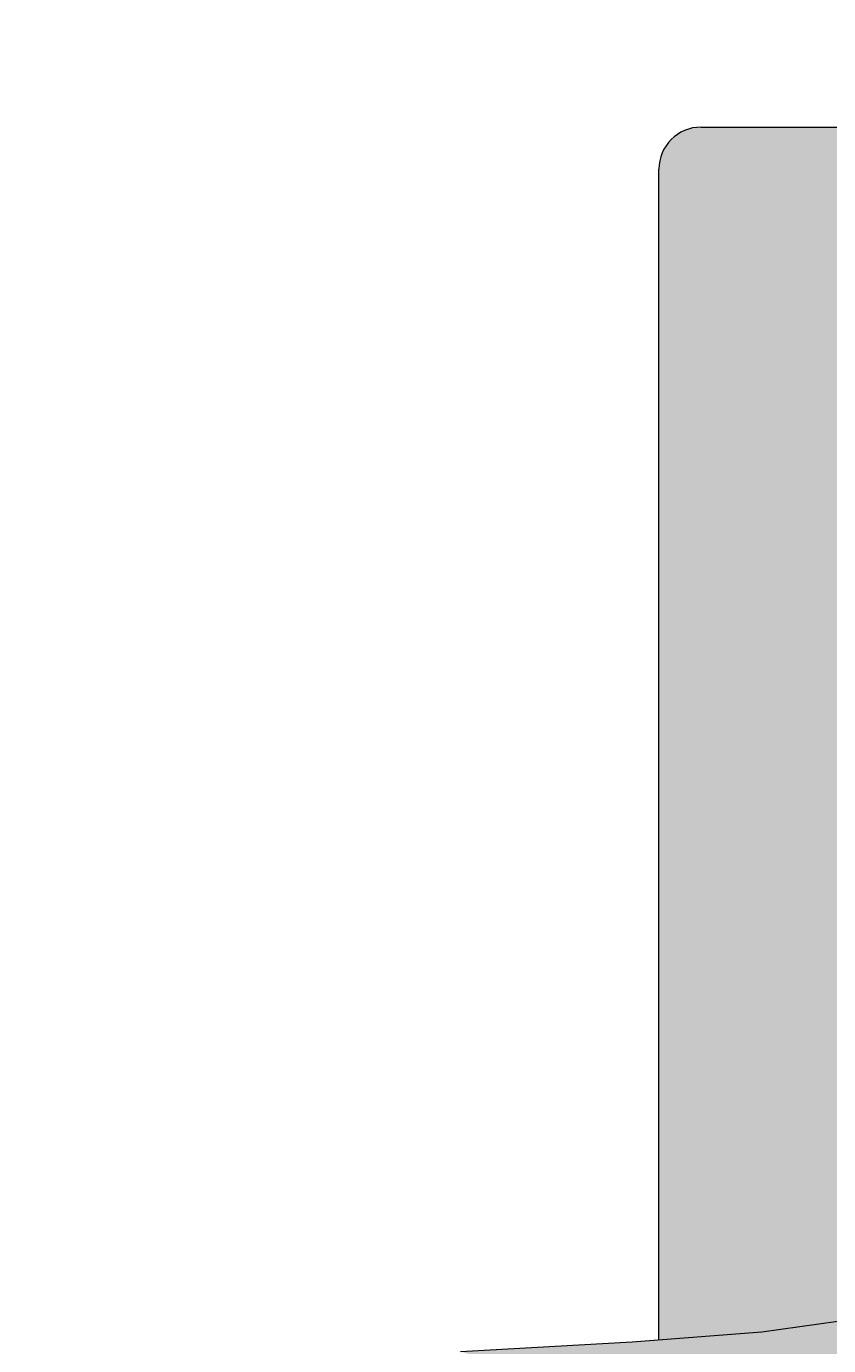
# Model space of a CAD drawing. Units: millimetres. Extents: x 27017497 to 27018854, y 7058029 to 7059154.
# Tile 73 of 91: x 27018360 to 27018390, y 7058174 to 7058224. Entities that reach past the tile are written whole.
import ezdxf

# ---------------------------------------------------------------- set-up
doc = ezdxf.new("R2010")
doc.units = ezdxf.units.MM
doc.layers.add('A-ANNO-DIMS', color=2, linetype='Continuous', lineweight=18)
doc.layers.add('A-FURN', color=8, linetype='Continuous', lineweight=18)
doc.layers.add('A-FURN-PATT', color=177, linetype='Continuous', lineweight=13, true_color=0x293189)
doc.styles.get("Standard").update_dxf_attribs({"font": 'arial.ttf'})
doc.dimstyles.get("Standard").update_dxf_attribs({"dimtxt": 0.18, "dimasz": 0.18, "dimexe": 0.18, "dimexo": 0.0625, "dimgap": 0.09, "dimtad": 0, "dimtih": 1, "dimtoh": 1, "dimdec": 4, "dimzin": 0, "dimdsep": 46, "dimtxsty": 'Standard', "dimcen": 0.09, "dimadec": 0, "dimazin": 0, "dimtfac": 1, "dimtdec": 4, "dimtofl": 0, "dimtmove": 0, "dimatfit": 3, "dimfxl": 1, "dimtolj": 1, "dimtzin": 0, "dimarcsym": 0})

# ---------------------------------------------------------------- blocks, each defined once
blk = doc.blocks.new('CAMMAT')
for p, q in [((0.65, -0.8204), (0.65, -1.93)), ((0.61, -1.97), (-0.61, -1.97))]:
    blk.add_line(p, q)
blk.add_lwpolyline([(0.8382, -0.8093), (0.6753, -0.8185), (0.5522, -0.828), (0.4622, -0.8406), (0.399, -0.8591), (0.356, -0.8862), (0.3267, -0.9248), (0.3046, -0.9777), (0.2832, -1.0476)])
blk.add_arc((0.61, -1.93), 0.04, 270, 360)
blk = doc.blocks.new('*D47')
at = {"layer": 'A-ANNO-DIMS', "color": 0, "lineweight": -2, "transparency": 16777216}
for p, q in [((27017561.166, 7058294.35), (27017561.166, 7058028.6)), ((27018790.606, 7058294.35), (27018790.606, 7058028.6)), ((27017561.346, 7058028.78), (27018175.431, 7058028.78)), ((27018790.426, 7058028.78), (27018176.341, 7058028.78))]:
    blk.add_line(p, q, dxfattribs=at)
at = {"layer": 'A-ANNO-DIMS', "color": 0, "transparency": 16777216}
for points in [[(27017561.346, 7058028.81), (27017561.346, 7058028.75), (27017561.166, 7058028.78)], [(27018790.426, 7058028.81), (27018790.426, 7058028.75), (27018790.606, 7058028.78)]]:
    blk.add_solid(points, dxfattribs=at)
at = {"layer": 'Defpoints', "color": 0, "transparency": 16777216}
for p in [(27017561.166, 7058294.412), (27018790.606, 7058294.412), (27018790.606, 7058028.78)]:
    blk.add_point(p, dxfattribs=at)
at = {"layer": 'A-ANNO-DIMS', "color": 0, "transparency": 16777216, "insert": (27018175.886, 7058028.78), "char_height": 0.18, "attachment_point": 5}
blk.add_mtext('\\A1;1229.4', dxfattribs=at)
blk = doc.blocks.new('*D48')
at = {"layer": 'A-ANNO-DIMS', "color": 0, "lineweight": -2, "transparency": 16777216}
for p, q in [((27018463.498, 7058622.912), (27017497.536, 7058622.912)), ((27017497.716, 7058622.732), (27017497.716, 7058357.753)), ((27017497.716, 7058092.41), (27017497.716, 7058357.389)), ((27018555.129, 7058092.23), (27017497.536, 7058092.23))]:
    blk.add_line(p, q, dxfattribs=at)
at = {"layer": 'A-ANNO-DIMS', "color": 0, "transparency": 16777216}
for points in [[(27017497.686, 7058622.732), (27017497.746, 7058622.732), (27017497.716, 7058622.912)], [(27017497.686, 7058092.41), (27017497.746, 7058092.41), (27017497.716, 7058092.23)]]:
    blk.add_solid(points, dxfattribs=at)
at = {"layer": 'Defpoints', "color": 0, "transparency": 16777216}
for p in [(27018463.561, 7058622.912), (27017497.716, 7058092.23), (27018555.192, 7058092.23)]:
    blk.add_point(p, dxfattribs=at)
at = {"layer": 'A-ANNO-DIMS', "color": 0, "transparency": 16777216, "insert": (27017497.716, 7058357.571), "char_height": 0.18, "attachment_point": 5}
blk.add_mtext('\\A1;530.7', dxfattribs=at)

msp = doc.modelspace()

# ---------------------------------------------------------------- hatches: boundary and pattern name
at = {"layer": 'A-FURN-PATT'}
h = msp.add_hatch(color=256, dxfattribs=at)
h.dxf.hatch_style = 1
h.paths.add_polyline_path([(27018435.86, 7058218.784, 0.414214), (27018434.267, 7058220.377), (27018385.674, 7058220.377, 0.414214), (27018384.081, 7058218.784), (27018384.081, 7058174.59), (27018387.977, 7058174.891), (27018391.56, 7058175.393), (27018394.078, 7058176.128), (27018395.791, 7058177.21), (27018396.958, 7058178.748), (27018397.838, 7058180.854), (27018398.69, 7058183.639), (27018399.293, 7058180.835), (27018399.836, 7058178.594), (27018400.426, 7058176.691), (27018401.17, 7058174.899), (27018402.177, 7058172.991), (27018403.552, 7058170.741), (27018405.403, 7058167.922), (27018407.838, 7058164.308), (27018410.273, 7058167.922), (27018412.124, 7058170.741), (27018413.499, 7058172.991), (27018414.506, 7058174.899), (27018415.25, 7058176.691), (27018415.84, 7058178.594), (27018416.383, 7058180.835), (27018416.986, 7058183.639), (27018417.838, 7058180.854), (27018418.718, 7058178.748), (27018419.885, 7058177.21), (27018421.598, 7058176.128), (27018424.116, 7058175.393), (27018427.699, 7058174.891), (27018432.604, 7058174.513), (27018435.86, 7058174.329)])
h.paths.add_polyline_path([(27018439.093, 7058174.146), (27018432.604, 7058174.513), (27018427.699, 7058174.891), (27018424.116, 7058175.393), (27018421.598, 7058176.128), (27018419.885, 7058177.21), (27018418.718, 7058178.748), (27018417.838, 7058180.854), (27018416.986, 7058183.639), (27018416.383, 7058180.835), (27018415.84, 7058178.594), (27018415.25, 7058176.691), (27018414.506, 7058174.899), (27018413.499, 7058172.991), (27018412.124, 7058170.741), (27018410.273, 7058167.922), (27018407.838, 7058164.308)])
h.paths.add_polyline_path([(27018403.552, 7058170.741), (27018402.177, 7058172.991), (27018401.17, 7058174.899), (27018400.426, 7058176.691), (27018399.836, 7058178.594), (27018399.293, 7058180.835), (27018398.69, 7058183.639), (27018397.838, 7058180.854), (27018396.958, 7058178.748), (27018395.791, 7058177.21), (27018394.078, 7058176.128), (27018391.56, 7058175.393), (27018387.977, 7058174.891), (27018383.071, 7058174.513), (27018376.583, 7058174.146), (27018407.838, 7058164.308), (27018405.403, 7058167.922)])
h.paths.add_polyline_path([(27018437.469, 7058173.635), (27018407.838, 7058164.308), (27018382.784, 7058172.194), (27018382.784, 7058162.502), (27018437.469, 7058162.502)])
h.paths.add_polyline_path([(27018435.86, 7058162.502), (27018384.081, 7058162.502), (27018384.081, 7058146.294, 0.414214), (27018385.674, 7058144.7), (27018434.267, 7058144.7, 0.414214), (27018435.86, 7058146.294)])
h.paths.add_polyline_path([(27018407.684, 7058159.418, -0.41419), (27018408.879, 7058158.223), (27018408.879, 7058148.664, -0.414237), (27018407.684, 7058147.469), (27018386.224, 7058147.469, -0.41419), (27018385.029, 7058148.663), (27018385.029, 7058158.223, -0.414237), (27018386.224, 7058159.418)], flags=16)
h.paths.add_polyline_path([(27018411.821, 7058159.418), (27018433.28, 7058159.418, -0.41419), (27018434.475, 7058158.223), (27018434.475, 7058148.664, -0.414237), (27018433.28, 7058147.469), (27018411.821, 7058147.469, -0.414214), (27018410.626, 7058148.664), (27018410.626, 7058158.223, -0.414214)], flags=16)
h.paths.add_polyline_path([(27018382.886, 7058160.632), (27018362.971, 7058160.632), (27018362.971, 7058144.7), (27018382.886, 7058144.7)])
h.paths.add_polyline_path([(27018379.136, 7058152.033, -1), (27018367.187, 7058152.033, -1)], flags=16)
h.paths.add_polyline_path([(27018376.861, 7058152.033, -1), (27018369.461, 7058152.033, -1)], flags=0)
h.paths.add_polyline_path([(27018456.97, 7058160.632), (27018437.055, 7058160.632), (27018437.055, 7058144.7), (27018456.97, 7058144.7)])
h.paths.add_polyline_path([(27018453.028, 7058152.033, -1), (27018441.079, 7058152.033, -1)], flags=16)
h.paths.add_polyline_path([(27018450.754, 7058152.033, -1), (27018443.354, 7058152.033, -1)], flags=0)
h.paths.add_polyline_path([(27018434.475, 7058158.223, 0.41419), (27018433.28, 7058159.418), (27018411.821, 7058159.418, 0.414214), (27018410.626, 7058158.223), (27018410.626, 7058148.664, 0.414214), (27018411.821, 7058147.469), (27018433.28, 7058147.469, 0.414237), (27018434.475, 7058148.664)], flags=0)

# ---------------------------------------------------------------- block references
at = {"layer": 'A-FURN', "xscale": 39.82996475819422, "yscale": 39.82996475819422, "zscale": 39.82996475819422, "rotation": 180}
msp.add_blockref('CAMMAT', (27018409.97, 7058141.912), dxfattribs=at)

# ---------------------------------------------------------------- dimensions: what is measured, and where the dimension line sits
at = {"layer": 'A-ANNO-DIMS'}
dim = msp.add_linear_dim(base=(27017497.716, 7058092.23), p1=(27018463.561, 7058622.912), p2=(27018555.192, 7058092.23), angle=90, dimstyle='Standard', override={"dimdec": 1, "dimlfac": 1, "dimrnd": 0, "dimzin": 0, "dimdsep": 46, "dimlunit": 2}, dxfattribs=at)
dim.commit()
dim.dimension.update_dxf_attribs({"geometry": '*D48', "text_midpoint": (27017497.716, 7058357.571)})
dim = msp.add_linear_dim(base=(27018790.606, 7058028.78), p1=(27017561.166, 7058294.412), p2=(27018790.606, 7058294.412), dimstyle='Standard', override={"dimdec": 1, "dimlfac": 1, "dimrnd": 0, "dimzin": 0, "dimdsep": 46, "dimlunit": 2}, dxfattribs=at)
dim.commit()
dim.dimension.update_dxf_attribs({"geometry": '*D47', "text_midpoint": (27018175.886, 7058028.78)})

doc.saveas('drawing.dxf')
